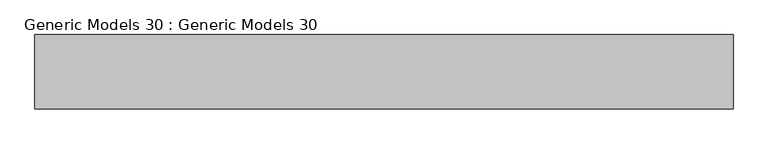
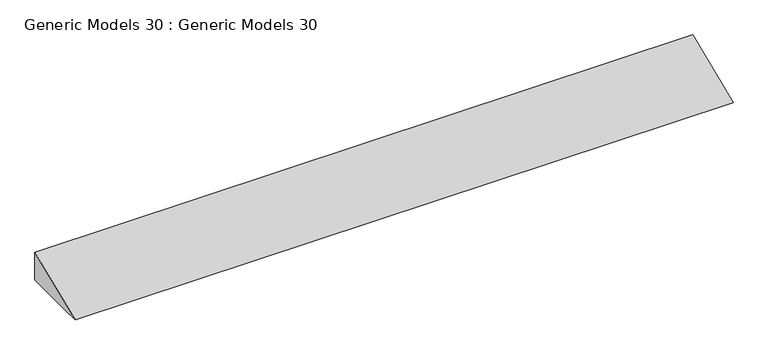
"""IFC4 building model written with IfcOpenShell, lengths in millimetres: proxy geometry, Generic Models 30 : Generic Models 30."""

from ifc_helpers import new_model, si_unit, frame, origin, place, context, project, spatial, polyline, outline, extrude, source, transform, mapped, element, save


def generic_models_30_generic_models_30_d6d6d2d1(model_context):
    return source(origin(), model_context, "Body", "SweptSolid", [
        extrude(outline(polyline([(-8681.2779205, 0.0), (-8878.1279205, 0.0), (-8147.9432518, 304.8), (-8147.9432518, 0.0), (-8681.2779205, 0.0)])), frame((-10006.8176097, 0.0, 0.0), z_axis=(1.0, 0.0, 0.0), x_axis=(0.0, 1.0, 0.0)), (0.0, 0.0, 1.0), 6872.2394833),
    ])


if __name__ == "__main__":
    model = new_model("IFC4")
    model_context = context("Model", 3, world=origin())
    ifc_project = project(units=[si_unit("LENGTHUNIT", "METRE", prefix="MILLI")], contexts=[model_context])
    site = spatial("IfcSite", under=ifc_project)
    building = spatial("IfcBuilding", under=site)
    placement = place(None, origin())
    generic_models_30_generic_models_30_shape = generic_models_30_generic_models_30_d6d6d2d1(model_context)
    element("IfcBuildingElementProxy", 1, Name="Generic Models 30 : Generic Models 30", ObjectType="Generic Models 30 : Generic Models 30", at=placement, inside=building, context=model_context, shape_type="MappedRepresentation", body=[
        mapped(generic_models_30_generic_models_30_shape, transform((0.0, 0.0, 0.0), x_axis=(1.0, 0.0, 0.0), y_axis=(0.0, 1.0, 0.0), z_axis=(0.0, 0.0, 1.0))),
    ])
    save(model, "model.ifc")
